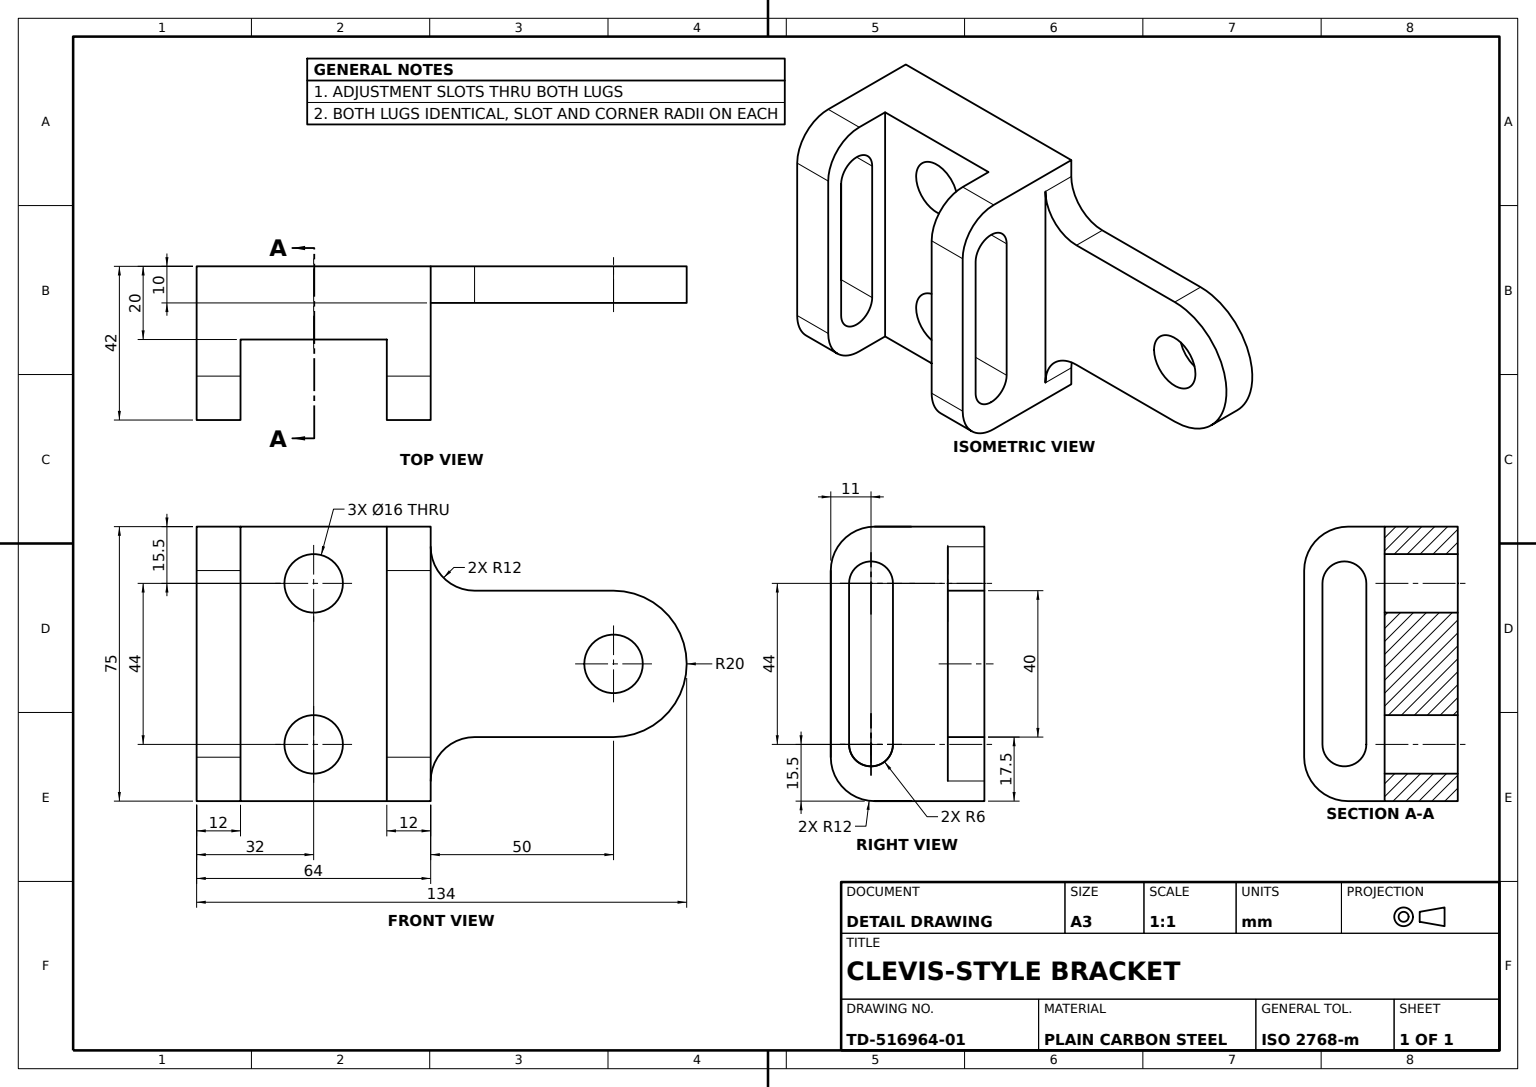
from build123d import *

# Parameters (mm, degrees)
BASE_BLOCK_SKETCH_W     = 64
BASE_BLOCK_SKETCH_H     = 75
BASE_BLOCK_DEPTH        = 20
CLAMP_LUG_A_SKETCH_W    = 12
CLAMP_LUG_A_SKETCH_H    = 75
CLAMP_LUG_A_DEPTH       = 22
CLAMP_LUG_B_SKETCH_W    = 12
CLAMP_LUG_B_SKETCH_H    = 75
CLAMP_LUG_B_DEPTH       = 22
ADJUSTMENT_SLOT_A_DEPTH = 101.463923873
ADJUSTMENT_SLOT_B_DEPTH = 101.463923873
MOUNTING_TAB_SKETCH_R   = 8
MOUNTING_TAB_DEPTH      = 10
BACK_WALL_CUT_SKETCH_R  = 8
BACK_WALL_CUT_DEPTH     = 156.128978595
LUG_A_EDGE_FILLET_R12_R = 12
LUG_B_EDGE_FILLET_R12_R = 12


with BuildPart() as part:
    # Base Block Sketch → Base Block (new body)
    with BuildSketch(Plane.XY):
        with Locations((32, 37.5)):
            Rectangle(BASE_BLOCK_SKETCH_W, BASE_BLOCK_SKETCH_H)
    extrude(amount=BASE_BLOCK_DEPTH)

    # Clamp Lug A Sketch → Clamp Lug A (add)
    with BuildSketch(Plane.XY.offset(20)):
        with Locations((6, 37.5)):
            Rectangle(CLAMP_LUG_A_SKETCH_W, CLAMP_LUG_A_SKETCH_H)
    extrude(amount=CLAMP_LUG_A_DEPTH)

    # Clamp Lug B Sketch → Clamp Lug B (add)
    with BuildSketch(Plane.XY.offset(20)):
        with Locations((58, 37.5)):
            Rectangle(CLAMP_LUG_B_SKETCH_W, CLAMP_LUG_B_SKETCH_H)
    extrude(amount=CLAMP_LUG_B_DEPTH)

    # Adjustment Slot A Sketch → Adjustment Slot A (cut, through all)
    with BuildSketch(Plane(origin=(12, 0, 0), x_dir=(0, 0, -1), z_dir=(1, 0, 0))):
        with BuildLine():
            Line((-37, 15.5), (-37, 59.5))
            ThreePointArc((-37, 59.5), (-31, 65.5), (-25, 59.5))
            Line((-25, 59.5), (-25, 15.5))
            ThreePointArc((-25, 15.5), (-31, 9.5), (-37, 15.5))
        make_face()
    extrude(amount=-ADJUSTMENT_SLOT_A_DEPTH, mode=Mode.SUBTRACT)

    # Adjustment Slot B Sketch → Adjustment Slot B (cut, through all)
    with BuildSketch(Plane.ZY.offset(-52)):
        with BuildLine():
            Line((25, 15.5), (25, 59.5))
            ThreePointArc((25, 59.5), (31, 65.5), (37, 59.5))
            Line((37, 59.5), (37, 15.5))
            ThreePointArc((37, 15.5), (31, 9.5), (25, 15.5))
        make_face()
    extrude(amount=-ADJUSTMENT_SLOT_B_DEPTH, mode=Mode.SUBTRACT)

    # Mounting Tab Sketch → Mounting Tab (add)
    with BuildSketch(Plane.XY):
        with BuildLine():
            Line((114, 57.5), (76, 57.5))
            ThreePointArc((76, 57.5), (67.514718626, 61.014718626), (64, 69.5))
            Line((64, 69.5), (64, 5.5))
            ThreePointArc((64, 5.5), (67.514718626, 13.985281374), (76, 17.5))
            Line((76, 17.5), (114, 17.5))
            ThreePointArc((114, 17.5), (134, 37.5), (114, 57.5))
        make_face()
        with Locations((114, 37.5)):
            Circle(MOUNTING_TAB_SKETCH_R, mode=Mode.SUBTRACT)
    extrude(amount=MOUNTING_TAB_DEPTH)

    # Back Wall Cut Sketch → Back Wall Cut (cut, through all)
    with BuildSketch(Plane.XY.offset(20)):
        with Locations((32, 59.5)):
            Circle(BACK_WALL_CUT_SKETCH_R)
        with Locations((32, 15.5)):
            Circle(BACK_WALL_CUT_SKETCH_R)
    extrude(amount=-BACK_WALL_CUT_DEPTH, mode=Mode.SUBTRACT)

    # Lug A Edge Fillet R12
    lug_a_edge_fillet_r12_edges = [part.edges().sort_by_distance(p)[0] for p in [
        (6, 0, 42),
        (6, 75, 42),
    ]]
    fillet(lug_a_edge_fillet_r12_edges, radius=LUG_A_EDGE_FILLET_R12_R)

    # Lug B Edge Fillet R12
    lug_b_edge_fillet_r12_edges = [part.edges().sort_by_distance(p)[0] for p in [
        (58, 0, 42),
        (58, 75, 42),
    ]]
    fillet(lug_b_edge_fillet_r12_edges, radius=LUG_B_EDGE_FILLET_R12_R)


solid = part.part
